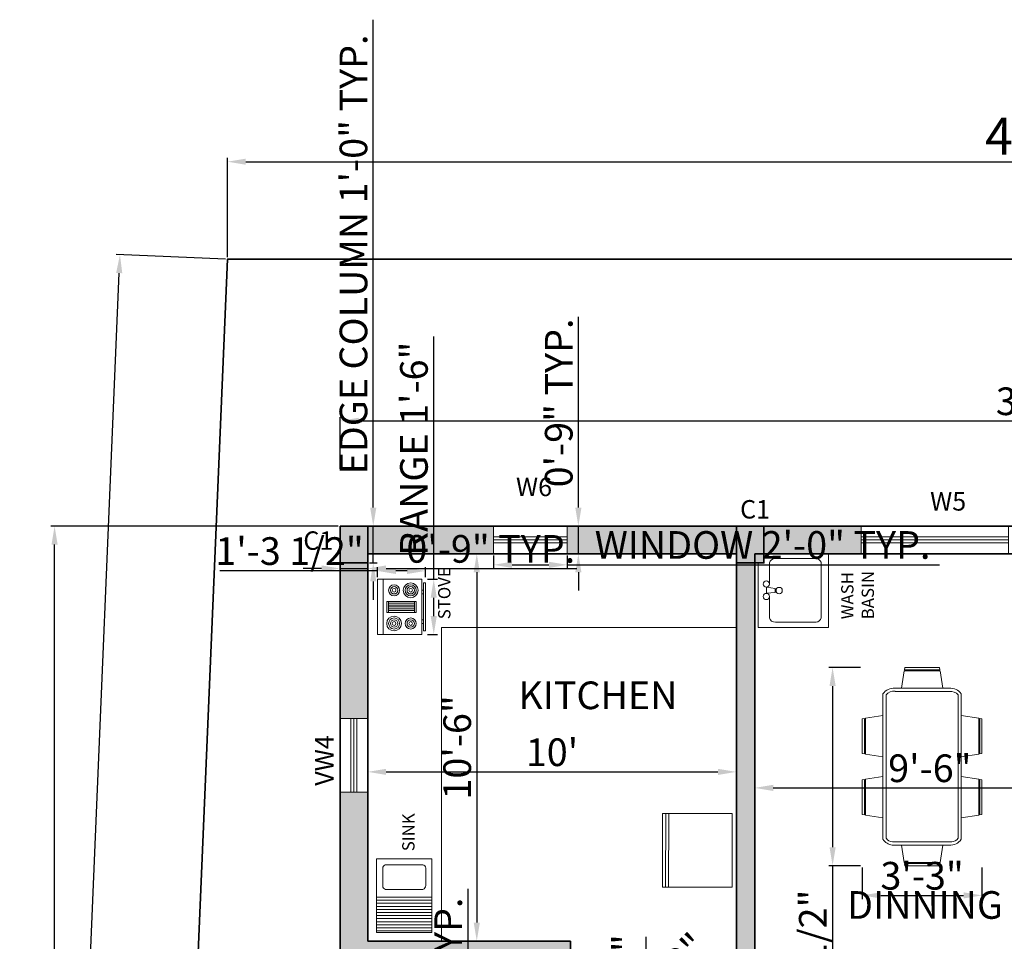
# Model space of a CAD drawing. Units: inches. Extents: x 4312 to 4955, y 6030 to 6717.
# Tile 4 of 5: x 4312 to 4632, y 6418 to 6717. Entities that reach past the tile are written whole.
import ezdxf

# ---------------------------------------------------------------- set-up
doc = ezdxf.new("R2010")
doc.units = ezdxf.units.IN
for name, color, linetype, lineweight in [('A-AREA-IDEN', 7, 'Continuous', 20), ('A-EQPM', 8, 'Continuous', 18), ('A-FLOR-CASE', 40, 'Continuous', 18), ('A-FLOR-FIXT', 9, 'Continuous', 18), ('A-FLOR-FIXT-PATT', 9, 'Continuous', 13), ('A-WALL', 7, 'Continuous', 35), ('C-PROP', 7, 'Continuous', 35), ('Dimensions', 112, 'Continuous', 13), ('Furniture', 30, 'Continuous', 18), ('Text', 30, 'Continuous', 18), ('Windows', 160, 'Continuous', 18)]:
    doc.layers.add(name, color=color, linetype=linetype, lineweight=lineweight)
doc.layers.add('A-WALL-PATT', color=251, linetype='Continuous', lineweight=13, true_color=0x636466)
doc.layers.add('Column', color=52, linetype='Continuous', lineweight=35, true_color=0xc8c92d)
doc.styles.get("Standard").update_dxf_attribs({"font": 'arial.ttf'})
doc.dimstyles.new('ISO-25', dxfattribs={"dimtxt": 9, "dimasz": 6, "dimexe": 1.25, "dimexo": 0.625, "dimtad": 1, "dimdec": 1, "dimlunit": 3, "dimtxsty": 'Standard', "dimcen": 2.5, "dimadec": 0, "dimazin": 0, "dimtfac": 1, "dimtdec": 1, "dimtmove": 0, "dimatfit": 3, "dimfxl": 1, "dimarcsym": 0})

# ---------------------------------------------------------------- blocks, each defined once
blk = doc.blocks.new('W')
at = {"layer": 'Windows'}
for p, q in [((4457.75, 6177.72), (4457.75, 6168.72)), ((4505.75, 6177.72), (4505.75, 6168.72)), ((4457.75, 6174.22), (4505.75, 6174.22)), ((4457.75, 6173.22), (4505.75, 6173.22)), ((4457.75, 6172.22), (4505.75, 6172.22))]:
    blk.add_line(p, q, dxfattribs=at)
blk = doc.blocks.new('KW')
at = {"layer": 'Windows'}
for p, q in [((4466.02, 6552.72), (4466.02, 6543.72)), ((4490.02, 6552.72), (4490.02, 6543.72)), ((4466.02, 6549.22), (4490.02, 6549.22)), ((4466.02, 6548.22), (4490.02, 6548.22)), ((4466.02, 6547.22), (4490.02, 6547.22))]:
    blk.add_line(p, q, dxfattribs=at)
blk = doc.blocks.new('*D9')
at = {"layer": 'Defpoints', "color": 0, "transparency": 16777216}
for p in [(4460.55, 6543.72), (4460.55, 6417.72), (4460.55, 6417.72)]:
    blk.add_point(p, dxfattribs=at)
at = {"layer": 'Dimensions', "color": 0, "lineweight": -2, "transparency": 16777216}
for p, q in [((4461.17, 6543.72), (4461.8, 6543.72)), ((4460.55, 6537.72), (4460.55, 6423.72)), ((4461.17, 6417.72), (4461.8, 6417.72))]:
    blk.add_line(p, q, dxfattribs=at)
at = {"layer": 'Dimensions', "color": 0, "transparency": 16777216}
for points in [[(4459.55, 6537.72), (4461.55, 6537.72), (4460.55, 6543.72)], [(4459.55, 6423.72), (4461.55, 6423.72), (4460.55, 6417.72)]]:
    blk.add_solid(points, dxfattribs=at)
at = {"layer": 'Dimensions', "color": 0, "transparency": 16777216, "insert": (4455.33, 6480.72), "char_height": 9, "attachment_point": 5, "rotation": 90}
blk.add_mtext('10\'-6"', dxfattribs=at)
blk = doc.blocks.new('*D10')
at = {"layer": 'Defpoints', "color": 0, "transparency": 16777216}
for p in [(4425.05, 6472.76), (4545.05, 6472.76), (4545.05, 6472.76)]:
    blk.add_point(p, dxfattribs=at)
at = {"layer": 'Dimensions', "color": 0, "lineweight": -2, "transparency": 16777216}
for p, q in [((4425.05, 6473.38), (4425.05, 6474.01)), ((4431.05, 6472.76), (4539.05, 6472.76)), ((4545.05, 6473.38), (4545.05, 6474.01))]:
    blk.add_line(p, q, dxfattribs=at)
at = {"layer": 'Dimensions', "color": 0, "transparency": 16777216}
for points in [[(4431.05, 6473.76), (4431.05, 6471.76), (4425.05, 6472.76)], [(4539.05, 6473.76), (4539.05, 6471.76), (4545.05, 6472.76)]]:
    blk.add_solid(points, dxfattribs=at)
at = {"layer": 'Dimensions', "color": 0, "transparency": 16777216, "insert": (4485.05, 6477.98), "char_height": 9, "attachment_point": 5}
blk.add_mtext("10'", dxfattribs=at)
blk = doc.blocks.new('*D11')
at = {"layer": 'Defpoints', "color": 0, "transparency": 16777216}
for p in [(4551.05, 6471.59), (4665.05, 6471.59), (4665.05, 6467.55)]:
    blk.add_point(p, dxfattribs=at)
at = {"layer": 'Dimensions', "color": 0, "lineweight": -2, "transparency": 16777216}
for p, q in [((4551.05, 6470.96), (4551.05, 6466.3)), ((4665.05, 6470.96), (4665.05, 6466.3)), ((4557.05, 6467.55), (4659.05, 6467.55))]:
    blk.add_line(p, q, dxfattribs=at)
at = {"layer": 'Dimensions', "color": 0, "transparency": 16777216}
for points in [[(4557.05, 6468.55), (4557.05, 6466.55), (4551.05, 6467.55)], [(4659.05, 6468.55), (4659.05, 6466.55), (4665.05, 6467.55)]]:
    blk.add_solid(points, dxfattribs=at)
at = {"layer": 'Dimensions', "color": 0, "transparency": 16777216, "insert": (4608.05, 6472.77), "char_height": 9, "attachment_point": 5}
blk.add_mtext('9\'-6"', dxfattribs=at)
blk = doc.blocks.new('Range-Oven - 30 in top')
for p, q in [((0, -3), (30, -3)), ((12, -6), (18, -6)), ((13, -20), (13, -6)), ((14, -6), (14, -20)), ((15, -20), (15, -6)), ((16, -6), (16, -20)), ((17, -20), (17, -6)), ((18, -20), (12, -20)), ((6, -24), (6, -25)), ((8, -25), (8, -24)), ((22, -25), (22, -24)), ((24, -24), (24, -25))]:
    blk.add_line(p, q)
for points in [[(0, -24), (0, 0), (30, 0), (30, -24)], [(12, -21), (12, -5), (18, -5), (18, -21)], [(2, -26), (2, -25), (28, -25), (28, -26)]]:
    blk.add_lwpolyline(points, close=True)
for centre, radius in [((6, -9), 4), ((6, -9), 3), ((6, -9), 2), ((6, -9), 1), ((24, -9), 3), ((24, -9), 2), ((24, -9), 1), ((6, -18), 3), ((6, -18), 2), ((24, -18), 4), ((24, -18), 3), ((24, -18), 2), ((6, -18), 1), ((24, -18), 1)]:
    blk.add_circle(centre, radius)
blk = doc.blocks.new('dinning')
for p, q in [((5019.18, 6524.81), (5018.3, 6519.14)), ((5019.18, 6524.81), (5030.85, 6524.81)), ((5019.35, 6525.87), (5019.24, 6525.17)), ((5030.79, 6525.17), (5019.24, 6525.17)), ((5019.35, 6525.87), (5030.68, 6525.87)), ((5030.79, 6525.17), (5030.68, 6525.87)), ((5031.73, 6519.14), (5030.85, 6524.81)), ((5039.01, 6524.81), (5038.13, 6519.14)), ((5039.02, 6524.81), (5050.68, 6524.81)), ((5039.18, 6525.87), (5039.07, 6525.17)), ((5050.62, 6525.17), (5039.07, 6525.17)), ((5039.18, 6525.87), (5050.51, 6525.87)), ((5050.62, 6525.17), (5050.51, 6525.87)), ((5051.56, 6519.14), (5050.68, 6524.81)), ((5058.57, 6519.15), (5011.29, 6519.15)), ((5058.25, 6518.15), (5011.62, 6518.15)), ((5003.77, 6512.23), (5009.43, 6513.11)), ((5009.43, 6515.21), (5009.43, 6497.59)), ((5010.43, 6515.26), (5010.43, 6497.59)), ((5059.43, 6496.76), (5059.43, 6516.04)), ((5060.43, 6496.7), (5060.43, 6515.21)), ((5066.1, 6512.23), (5060.43, 6513.11)), ((5002.7, 6512.06), (5003.41, 6512.17)), ((5002.7, 6512.06), (5002.7, 6500.73)), ((5003.41, 6500.62), (5003.41, 6512.17)), ((5003.77, 6512.23), (5003.77, 6500.56)), ((5066.09, 6512.23), (5066.09, 6500.56)), ((5067.16, 6512.06), (5066.45, 6512.17)), ((5066.45, 6500.62), (5066.45, 6512.17)), ((5067.16, 6512.06), (5067.16, 6500.73)), ((5003.41, 6500.62), (5002.7, 6500.73)), ((5009.43, 6499.68), (5003.77, 6500.56)), ((5060.43, 6499.68), (5066.09, 6500.56)), ((5066.45, 6500.62), (5067.16, 6500.73)), ((5011.62, 6494.65), (5058.25, 6494.65)), ((5011.29, 6493.65), (5058.57, 6493.65)), ((5019.18, 6487.98), (5018.3, 6493.65)), ((5031.73, 6493.65), (5030.85, 6487.98)), ((5039.01, 6487.98), (5038.13, 6493.65)), ((5051.56, 6493.65), (5050.68, 6487.98)), ((5019.18, 6487.98), (5030.85, 6487.98)), ((5019.35, 6486.92), (5019.24, 6487.63)), ((5030.79, 6487.63), (5019.24, 6487.63)), ((5030.79, 6487.63), (5030.68, 6486.92)), ((5039.02, 6487.98), (5050.68, 6487.98)), ((5039.18, 6486.92), (5039.07, 6487.63)), ((5050.62, 6487.63), (5039.07, 6487.63)), ((5050.62, 6487.63), (5050.51, 6486.92)), ((5019.35, 6486.92), (5030.68, 6486.92)), ((5039.18, 6486.92), (5050.51, 6486.92))]:
    blk.add_line(p, q)
for centre, radius, start, end in [((5013.59, 6515.65), 4.18, 123.3176, 186.0843), ((5013.59, 6515.65), 3.18, 128.372, 186.976), ((5056.27, 6515.65), 3.18, 6.976, 51.628), ((5056.27, 6515.65), 4.18, 353.9157, 56.6824), ((5013.59, 6497.14), 4.18, 173.9157, 236.6824), ((5013.61, 6497.16), 3.21, 172.3391, 231.5588), ((5056.27, 6497.14), 3.18, 308.372, 353.024), ((5056.27, 6497.14), 4.18, 303.3176, 353.9157)]:
    blk.add_arc(centre, radius, start, end)
blk = doc.blocks.new('*D38')
at = {"layer": 'Defpoints', "color": 0, "transparency": 16777216}
for p in [(4860.05, 6586.94), (4416.05, 6570.77), (4860.05, 6570.77)]:
    blk.add_point(p, dxfattribs=at)
at = {"layer": 'Dimensions', "color": 0, "lineweight": -2, "transparency": 16777216}
for p, q in [((4416.05, 6571.39), (4416.05, 6588.19)), ((4422.05, 6586.94), (4854.05, 6586.94)), ((4860.05, 6571.39), (4860.05, 6588.19))]:
    blk.add_line(p, q, dxfattribs=at)
at = {"layer": 'Dimensions', "color": 0, "transparency": 16777216}
for points in [[(4422.05, 6587.94), (4422.05, 6585.94), (4416.05, 6586.94)], [(4854.05, 6587.94), (4854.05, 6585.94), (4860.05, 6586.94)]]:
    blk.add_solid(points, dxfattribs=at)
at = {"layer": 'Dimensions', "color": 0, "transparency": 16777216, "insert": (4638.05, 6592.16), "char_height": 9, "attachment_point": 5}
blk.add_mtext("37'", dxfattribs=at)
blk = doc.blocks.new('*D40')
at = {"layer": 'Defpoints', "color": 0, "transparency": 16777216}
for p in [(4895.36, 6671.27), (4379.36, 6639.55), (4895.36, 6639.55)]:
    blk.add_point(p, dxfattribs=at)
at = {"layer": 'Dimensions', "color": 0, "lineweight": -2, "transparency": 16777216}
for p, q in [((4379.36, 6640.17), (4379.36, 6672.52)), ((4385.36, 6671.27), (4889.36, 6671.27)), ((4895.36, 6640.17), (4895.36, 6672.52))]:
    blk.add_line(p, q, dxfattribs=at)
at = {"layer": 'Dimensions', "color": 0, "transparency": 16777216}
for points in [[(4385.36, 6672.27), (4385.36, 6670.27), (4379.36, 6671.27)], [(4889.36, 6672.27), (4889.36, 6670.27), (4895.36, 6671.27)]]:
    blk.add_solid(points, dxfattribs=at)
at = {"layer": 'Dimensions', "color": 0, "transparency": 16777216, "insert": (4637.36, 6678.02), "char_height": 12, "attachment_point": 5}
blk.add_mtext("43'", dxfattribs=at)
blk = doc.blocks.new('*D43')
at = {"layer": 'Defpoints', "color": 0, "transparency": 16777216}
for p in [(4344.4, 6641.02), (4379.36, 6639.55), (4355.36, 6070.55)]:
    blk.add_point(p, dxfattribs=at)
at = {"layer": 'Dimensions', "color": 0, "lineweight": -2, "transparency": 16777216}
for p, q in [((4378.74, 6639.57), (4343.16, 6641.08)), ((4320.66, 6078.02), (4344.15, 6635.03)), ((4354.74, 6070.57), (4319.16, 6072.08))]:
    blk.add_line(p, q, dxfattribs=at)
at = {"layer": 'Dimensions', "color": 0, "transparency": 16777216}
for points in [[(4343.15, 6635.07), (4345.15, 6634.99), (4344.4, 6641.02)], [(4319.66, 6078.06), (4321.66, 6077.98), (4320.4, 6072.02)]]:
    blk.add_solid(points, dxfattribs=at)
at = {"layer": 'Dimensions', "color": 0, "transparency": 16777216, "insert": (4325.68, 6356.81), "char_height": 12, "attachment_point": 5, "rotation": 87.5847}
blk.add_mtext('47\'-5.5"', dxfattribs=at)
blk = doc.blocks.new('COLUMN-9X12-EDGE')
h = blk.add_hatch(color=256)
h.dxf.hatch_style = 1
h.paths.add_polyline_path([(9, 12), (0, 12), (0, 0), (9, 0)])
blk.add_lwpolyline([(9, 0), (0, 0)])
blk = doc.blocks.new('*D53')
at = {"layer": 'Defpoints', "color": 0, "transparency": 16777216}
for p in [(4425.05, 6552.72), (4426.85, 6552.72), (4425.05, 6540.72)]:
    blk.add_point(p, dxfattribs=at)
at = {"layer": 'Dimensions', "color": 0, "lineweight": -2, "transparency": 16777216}
for p, q in [((4426.85, 6558.72), (4426.85, 6717.46)), ((4425.67, 6552.72), (4428.1, 6552.72)), ((4426.85, 6540.72), (4426.85, 6552.72)), ((4425.67, 6540.72), (4428.1, 6540.72)), ((4426.85, 6534.72), (4426.85, 6528.72))]:
    blk.add_line(p, q, dxfattribs=at)
at = {"layer": 'Dimensions', "color": 0, "transparency": 16777216}
for points in [[(4425.85, 6558.72), (4427.85, 6558.72), (4426.85, 6552.72)], [(4425.85, 6534.72), (4427.85, 6534.72), (4426.85, 6540.72)]]:
    blk.add_solid(points, dxfattribs=at)
at = {"layer": 'Dimensions', "color": 0, "transparency": 16777216, "insert": (4421.57, 6641.09), "char_height": 9, "attachment_point": 5, "rotation": 90}
blk.add_mtext('EDGE COLUMN 1\'-0" TYP.', dxfattribs=at)
blk = doc.blocks.new('*D54')
at = {"layer": 'Defpoints', "color": 0, "transparency": 16777216}
for p in [(4416.05, 6540.72), (4425.05, 6540.72), (4425.05, 6538.92)]:
    blk.add_point(p, dxfattribs=at)
at = {"layer": 'Dimensions', "color": 0, "lineweight": -2, "transparency": 16777216}
for p, q in [((4410.05, 6538.92), (4404.05, 6538.92)), ((4416.05, 6540.1), (4416.05, 6537.67)), ((4416.05, 6538.92), (4425.05, 6538.92)), ((4425.05, 6540.1), (4425.05, 6537.67)), ((4431.05, 6538.92), (4493.16, 6538.92))]:
    blk.add_line(p, q, dxfattribs=at)
at = {"layer": 'Dimensions', "color": 0, "transparency": 16777216}
for points in [[(4410.05, 6539.92), (4410.05, 6537.92), (4416.05, 6538.92)], [(4431.05, 6539.92), (4431.05, 6537.92), (4425.05, 6538.92)]]:
    blk.add_solid(points, dxfattribs=at)
at = {"layer": 'Dimensions', "color": 0, "transparency": 16777216, "insert": (4465.1, 6544.14), "char_height": 9, "attachment_point": 5}
blk.add_mtext('0\'-9" TYP.', dxfattribs=at)
blk = doc.blocks.new('*D63')
at = {"layer": 'Defpoints', "color": 0, "transparency": 16777216}
for p in [(4466.02, 6543.72), (4490.02, 6543.72), (4490.02, 6540.12)]:
    blk.add_point(p, dxfattribs=at)
at = {"layer": 'Dimensions', "color": 0, "lineweight": -2, "transparency": 16777216}
for p, q in [((4466.02, 6543.1), (4466.02, 6538.87)), ((4490.02, 6543.1), (4490.02, 6538.87)), ((4472.02, 6540.12), (4484.02, 6540.12)), ((4490.02, 6540.12), (4611.16, 6540.12))]:
    blk.add_line(p, q, dxfattribs=at)
at = {"layer": 'Dimensions', "color": 0, "transparency": 16777216}
for points in [[(4472.02, 6541.12), (4472.02, 6539.12), (4466.02, 6540.12)], [(4484.02, 6541.12), (4484.02, 6539.12), (4490.02, 6540.12)]]:
    blk.add_solid(points, dxfattribs=at)
at = {"layer": 'Dimensions', "color": 0, "transparency": 16777216, "insert": (4553.59, 6545.41), "char_height": 9, "attachment_point": 5}
blk.add_mtext('WINDOW 2\'-0" TYP.', dxfattribs=at)
blk = doc.blocks.new('*D64')
at = {"layer": 'Defpoints', "color": 0, "transparency": 16777216}
for p in [(4490.02, 6552.72), (4493.62, 6552.72), (4490.02, 6543.72)]:
    blk.add_point(p, dxfattribs=at)
at = {"layer": 'Dimensions', "color": 0, "lineweight": -2, "transparency": 16777216}
for p, q in [((4493.62, 6558.72), (4493.62, 6620.83)), ((4490.65, 6552.72), (4494.87, 6552.72)), ((4493.62, 6543.72), (4493.62, 6552.72)), ((4490.65, 6543.72), (4494.87, 6543.72)), ((4493.62, 6537.72), (4493.62, 6531.72))]:
    blk.add_line(p, q, dxfattribs=at)
at = {"layer": 'Dimensions', "color": 0, "transparency": 16777216}
for points in [[(4492.62, 6558.72), (4494.62, 6558.72), (4493.62, 6552.72)], [(4492.62, 6537.72), (4494.62, 6537.72), (4493.62, 6543.72)]]:
    blk.add_solid(points, dxfattribs=at)
at = {"layer": 'Dimensions', "color": 0, "transparency": 16777216, "insert": (4488.4, 6592.78), "char_height": 9, "attachment_point": 5, "rotation": 90}
blk.add_mtext('0\'-9" TYP.', dxfattribs=at)
blk = doc.blocks.new('*D70')
at = {"layer": 'Defpoints', "color": 0, "transparency": 16777216}
for p in [(4512.05, 6387.72), (4515.65, 6387.72), (4512.05, 6363.72)]:
    blk.add_point(p, dxfattribs=at)
at = {"layer": 'Dimensions', "color": 0, "lineweight": -2, "transparency": 16777216}
for p, q in [((4515.65, 6387.72), (4515.65, 6419.05)), ((4512.67, 6387.72), (4516.9, 6387.72)), ((4515.65, 6369.72), (4515.65, 6381.72)), ((4512.67, 6363.72), (4516.9, 6363.72))]:
    blk.add_line(p, q, dxfattribs=at)
at = {"layer": 'Dimensions', "color": 0, "transparency": 16777216}
for points in [[(4514.65, 6381.72), (4516.65, 6381.72), (4515.65, 6387.72)], [(4514.65, 6369.72), (4516.65, 6369.72), (4515.65, 6363.72)]]:
    blk.add_solid(points, dxfattribs=at)
at = {"layer": 'Dimensions', "color": 0, "transparency": 16777216, "insert": (4510.43, 6406.39), "char_height": 9, "attachment_point": 5, "rotation": 90}
blk.add_mtext('2\'-0"', dxfattribs=at)
blk = doc.blocks.new('*D73')
at = {"layer": 'Defpoints', "color": 0, "transparency": 16777216}
for p in [(4447.05, 6327.89), (4457.7, 6327.89), (4447.05, 6256.83)]:
    blk.add_point(p, dxfattribs=at)
at = {"layer": 'Dimensions', "color": 0, "lineweight": -2, "transparency": 16777216}
for p, q in [((4457.7, 6327.89), (4457.7, 6434.68)), ((4447.67, 6327.89), (4458.95, 6327.89)), ((4457.7, 6262.83), (4457.7, 6321.89)), ((4447.67, 6256.83), (4458.95, 6256.83))]:
    blk.add_line(p, q, dxfattribs=at)
at = {"layer": 'Dimensions', "color": 0, "transparency": 16777216}
for points in [[(4456.7, 6321.89), (4458.7, 6321.89), (4457.7, 6327.89)], [(4456.7, 6262.83), (4458.7, 6262.83), (4457.7, 6256.83)]]:
    blk.add_solid(points, dxfattribs=at)
at = {"layer": 'Dimensions', "color": 0, "transparency": 16777216, "insert": (4452.42, 6384.28), "char_height": 9, "attachment_point": 5, "rotation": 90}
blk.add_mtext('SOFA 5\'-11" TYP.', dxfattribs=at)
blk = doc.blocks.new('*D81')
at = {"layer": 'Defpoints', "color": 0, "transparency": 16777216}
for p in [(4443.84, 6535.43), (4446.54, 6535.43), (4443.84, 6517.43)]:
    blk.add_point(p, dxfattribs=at)
at = {"layer": 'Dimensions', "color": 0, "lineweight": -2, "transparency": 16777216}
for p, q in [((4446.54, 6535.43), (4446.54, 6614.35)), ((4444.47, 6535.43), (4447.79, 6535.43)), ((4446.54, 6523.43), (4446.54, 6529.43)), ((4444.47, 6517.43), (4447.79, 6517.43))]:
    blk.add_line(p, q, dxfattribs=at)
at = {"layer": 'Dimensions', "color": 0, "transparency": 16777216}
for points in [[(4445.54, 6529.43), (4447.54, 6529.43), (4446.54, 6535.43)], [(4445.54, 6523.43), (4447.54, 6523.43), (4446.54, 6517.43)]]:
    blk.add_solid(points, dxfattribs=at)
at = {"layer": 'Dimensions', "color": 0, "transparency": 16777216, "insert": (4441.26, 6577.89), "char_height": 9, "attachment_point": 5, "rotation": 90}
blk.add_mtext('RANGE 1\'-6"', dxfattribs=at)
blk = doc.blocks.new('*D82')
at = {"layer": 'Defpoints', "color": 0, "transparency": 16777216}
for p in [(4428.24, 6538.13), (4428.24, 6535.43), (4443.84, 6535.43)]:
    blk.add_point(p, dxfattribs=at)
at = {"layer": 'Dimensions', "color": 0, "lineweight": -2, "transparency": 16777216}
for p, q in [((4428.24, 6536.06), (4428.24, 6539.38)), ((4443.84, 6536.06), (4443.84, 6539.38)), ((4428.24, 6538.13), (4376.94, 6538.13)), ((4437.84, 6538.13), (4434.24, 6538.13))]:
    blk.add_line(p, q, dxfattribs=at)
at = {"layer": 'Dimensions', "color": 0, "transparency": 16777216}
for points in [[(4434.24, 6539.13), (4434.24, 6537.13), (4428.24, 6538.13)], [(4437.84, 6539.13), (4437.84, 6537.13), (4443.84, 6538.13)]]:
    blk.add_solid(points, dxfattribs=at)
at = {"layer": 'Dimensions', "color": 0, "transparency": 16777216, "insert": (4399.59, 6543.42), "char_height": 9, "attachment_point": 5}
blk.add_mtext('1\'-3 1/2"', dxfattribs=at)
blk = doc.blocks.new('*D83')
at = {"layer": 'Defpoints', "color": 0, "transparency": 16777216}
for p in [(4586.05, 6506.69), (4576.38, 6442.24), (4586.05, 6442.24)]:
    blk.add_point(p, dxfattribs=at)
at = {"layer": 'Dimensions', "color": 0, "lineweight": -2, "transparency": 16777216}
for p, q in [((4585.42, 6506.69), (4575.13, 6506.69)), ((4576.38, 6500.69), (4576.38, 6448.24)), ((4585.42, 6442.24), (4575.13, 6442.24)), ((4576.38, 6442.24), (4576.38, 6315.1))]:
    blk.add_line(p, q, dxfattribs=at)
at = {"layer": 'Dimensions', "color": 0, "transparency": 16777216}
for points in [[(4575.38, 6500.69), (4577.38, 6500.69), (4576.38, 6506.69)], [(4575.38, 6448.24), (4577.38, 6448.24), (4576.38, 6442.24)]]:
    blk.add_solid(points, dxfattribs=at)
at = {"layer": 'Dimensions', "color": 0, "transparency": 16777216, "insert": (4571.1, 6375.67), "char_height": 9, "attachment_point": 5, "rotation": 90}
blk.add_mtext('DINING SET 5\'-4 1/2"', dxfattribs=at)
blk = doc.blocks.new('*D84')
at = {"layer": 'Defpoints', "color": 0, "transparency": 16777216}
for p in [(4586.05, 6442.24), (4625, 6442.24), (4625, 6432.57)]:
    blk.add_point(p, dxfattribs=at)
at = {"layer": 'Dimensions', "color": 0, "lineweight": -2, "transparency": 16777216}
for p, q in [((4586.05, 6441.61), (4586.05, 6431.32)), ((4625, 6441.61), (4625, 6431.32)), ((4592.05, 6432.57), (4619, 6432.57))]:
    blk.add_line(p, q, dxfattribs=at)
at = {"layer": 'Dimensions', "color": 0, "transparency": 16777216}
for points in [[(4592.05, 6433.57), (4592.05, 6431.57), (4586.05, 6432.57)], [(4619, 6433.57), (4619, 6431.57), (4625, 6432.57)]]:
    blk.add_solid(points, dxfattribs=at)
at = {"layer": 'Dimensions', "color": 0, "transparency": 16777216, "insert": (4605.52, 6437.79), "char_height": 9, "attachment_point": 5}
blk.add_mtext('3\'-3"', dxfattribs=at)
blk = doc.blocks.new('*D90')
at = {"layer": 'Defpoints', "color": 0, "transparency": 16777216}
for p in [(4323.11, 6552.72), (4416.05, 6552.72), (4368.05, 6087.72)]:
    blk.add_point(p, dxfattribs=at)
at = {"layer": 'Dimensions', "color": 0, "lineweight": -2, "transparency": 16777216}
for p, q in [((4415.42, 6552.72), (4321.86, 6552.72)), ((4323.11, 6093.72), (4323.11, 6546.72)), ((4367.42, 6087.72), (4321.86, 6087.72))]:
    blk.add_line(p, q, dxfattribs=at)
at = {"layer": 'Dimensions', "color": 0, "transparency": 16777216}
for points in [[(4322.11, 6546.72), (4324.11, 6546.72), (4323.11, 6552.72)], [(4322.11, 6093.72), (4324.11, 6093.72), (4323.11, 6087.72)]]:
    blk.add_solid(points, dxfattribs=at)
at = {"layer": 'Dimensions', "color": 0, "transparency": 16777216, "insert": (4317.89, 6320.22), "char_height": 9, "attachment_point": 5, "rotation": 90}
blk.add_mtext('38\'-9"', dxfattribs=at)
blk = doc.blocks.new('*D97')
at = {"layer": 'Defpoints', "color": 0, "transparency": 16777216}
for p in [(4505.02, 6380.69), (4488.05, 6363.72)]:
    blk.add_point(p, dxfattribs=at)
at = {"layer": 'Dimensions', "color": 0, "lineweight": -2, "transparency": 16777216}
for p, q in [((4537.4, 6413.07), (4509.26, 6384.94)), ((4488.05, 6363.72), (4505.02, 6380.69))]:
    blk.add_line(p, q, dxfattribs=at)
at = {"layer": 'Dimensions', "color": 0, "transparency": 16777216}
blk.add_solid([(4508.56, 6385.64), (4509.97, 6384.23), (4505.02, 6380.69)], dxfattribs=at)
at = {"layer": 'Dimensions', "color": 0, "transparency": 16777216, "insert": (4521.76, 6404.82), "char_height": 9, "attachment_point": 5, "rotation": 44.9998}
blk.add_mtext('R2\'-0"', dxfattribs=at)

msp = doc.modelspace()

# ---------------------------------------------------------------- hatches: boundary and pattern name
at = {"layer": 'A-FLOR-FIXT-PATT'}
h = msp.add_hatch(dxfattribs=at)
h.set_pattern_fill('ANSI31', color=256, scale=0.314961, angle=-45, style=0)
h.paths.add_polyline_path([(4427.93, 6420.52), (4445.93, 6420.52), (4445.93, 6432.52), (4427.93, 6432.52)])
at = {"layer": 'A-WALL-PATT'}
h = msp.add_hatch(color=256, dxfattribs=at)
h.dxf.hatch_style = 1
h.paths.add_polyline_path([(4466.02, 6552.72), (4425.05, 6552.72), (4425.05, 6543.72), (4466.02, 6543.72)])
h = msp.add_hatch(color=256, dxfattribs=at)
h.dxf.hatch_style = 1
h.paths.add_polyline_path([(4545.13, 6552.72), (4490.02, 6552.72), (4490.02, 6543.72), (4545.13, 6543.72)])
h = msp.add_hatch(color=256, dxfattribs=at)
h.dxf.hatch_style = 1
h.paths.add_polyline_path([(4585.64, 6552.72), (4554.13, 6552.72), (4554.13, 6543.72), (4585.64, 6543.72)])
h = msp.add_hatch(color=256, dxfattribs=at)
h.dxf.hatch_style = 1
h.paths.add_polyline_path([(4425.05, 6540.72), (4416.05, 6540.72), (4416.05, 6490.16), (4425.05, 6490.16)])
h = msp.add_hatch(color=256, dxfattribs=at)
h.dxf.hatch_style = 1
h.paths.add_polyline_path([(4551.05, 6540.72), (4545.05, 6540.72), (4545.05, 6411.72), (4551.05, 6411.72)])
h = msp.add_hatch(color=256, dxfattribs=at)
h.dxf.hatch_style = 1
h.paths.add_polyline_path([(4425.05, 6466.16), (4416.05, 6466.16), (4416.05, 6392.17), (4425.05, 6392.17), (4425.05, 6411.72), (4485.05, 6411.72), (4485.05, 6387.72), (4491.05, 6387.72), (4491.05, 6417.72), (4425.05, 6417.72)])
at = {"layer": 'Column'}
h = msp.add_hatch(color=256, dxfattribs=at)
h.dxf.hatch_style = 1
h.paths.add_polyline_path([(4554.05, 6540.72), (4554.05, 6543.72), (4554.05, 6552.72), (4545.05, 6552.72), (4545.05, 6540.72), (4551.05, 6540.72)])

# ---------------------------------------------------------------- linework, layer by layer
at = {"layer": 'A-EQPM'}
for p, q in [((4521.05, 6459.2), (4521, 6435.2)), ((4543.67, 6459.2), (4521.05, 6459.2)), ((4522.05, 6459.2), (4522, 6435.2)), ((4523.05, 6459.2), (4523, 6435.2)), ((4543.67, 6459.2), (4543.67, 6435.2)), ((4545.05, 6459.2), (4545.05, 6459.2)), ((4521, 6435.2), (4543.67, 6435.2))]:
    msp.add_line(p, q, dxfattribs=at)
at = {"layer": 'A-FLOR-CASE'}
for p, q in [((4575.05, 6519.72), (4575.05, 6543.72)), ((4552.19, 6540.72), (4552.19, 6519.72)), ((4449.05, 6417.72), (4449.05, 6519.72)), ((4449.05, 6519.72), (4545.05, 6519.72)), ((4552.19, 6519.72), (4575.05, 6519.72))]:
    msp.add_line(p, q, dxfattribs=at)
at = {"layer": 'A-FLOR-FIXT'}
for points in [[(4570.94, 6542.18), (4557.61, 6542.18, 0.355496), (4555.86, 6540.75), (4555.86, 6533.87)], [(4555.86, 6529.82), (4555.86, 6522.89, 0.38014), (4557.77, 6521.47), (4571.02, 6521.47, 0.335385), (4572.63, 6522.9), (4572.63, 6540.95, 0.335385), (4570.86, 6542.18)]]:
    msp.add_lwpolyline(points, format="xyb", dxfattribs=at)
for points in [[(4554.84, 6530.85), (4557.69, 6531.12), (4557.69, 6532.46), (4554.84, 6532.85)], [(4427.93, 6420.52), (4427.93, 6444.52), (4445.93, 6444.52), (4445.93, 6420.52)]]:
    msp.add_lwpolyline(points, close=True, dxfattribs=at)
msp.add_lwpolyline([(4442.97, 6434.52, 0.38014), (4443.93, 6435.81), (4443.93, 6441.44, 0.335385), (4442.96, 6442.52), (4430.76, 6442.52, 0.335385), (4429.93, 6441.33), (4429.93, 6435.71, 0.355496), (4430.89, 6434.52)], format="xyb", close=True, dxfattribs=at)
for centre in [(4554.84, 6533.87), (4558.98, 6531.75), (4554.84, 6529.82)]:
    msp.add_circle(centre, 1.02, dxfattribs=at)
at = {"layer": 'A-WALL'}
for p, q in [((4416.05, 6223.72), (4416.05, 6552.72)), ((4416.05, 6552.72), (4860.05, 6552.72)), ((4425.05, 6417.72), (4425.05, 6552.72)), ((4545.05, 6552.72), (4545.05, 6411.72)), ((4425.05, 6543.72), (4545.05, 6543.72)), ((4551.05, 6543.72), (4551.05, 6411.72)), ((4551.05, 6543.72), (4851.05, 6543.72)), ((4425.05, 6417.72), (4491.05, 6417.72)), ((4491.05, 6387.72), (4491.05, 6417.72))]:
    msp.add_line(p, q, dxfattribs=at)
at = {"layer": 'C-PROP'}
msp.add_lwpolyline([(4895.36, 6639.55), (4895.36, 6070.55), (4355.36, 6070.55), (4379.36, 6639.55)], close=True, dxfattribs=at)
at = {"layer": 'Column'}
msp.add_lwpolyline([(4554.05, 6552.72), (4554.05, 6540.72), (4545.05, 6540.72)], dxfattribs=at)

# ---------------------------------------------------------------- block references
at = {"layer": 'A-EQPM', "xscale": 0.6, "yscale": 0.6, "zscale": 0.6, "rotation": 90}
msp.add_blockref('Range-Oven - 30 in top', (4428.24, 6517.43), dxfattribs=at)
at = {"layer": 'Column'}
msp.add_blockref('COLUMN-9X12-EDGE', (4416.05, 6540.72), dxfattribs=at)
at = {"layer": 'Furniture', "rotation": 270}
msp.add_blockref('dinning', (-1900.87, 11509.39), dxfattribs=at)
at = {"layer": 'Windows'}
for name, p in [('KW', (0, 0)), ('W', (127.88, 375))]:
    msp.add_blockref(name, p, dxfattribs=at)
at = {"layer": 'Windows', "rotation": 270}
msp.add_blockref('KW', (-2127.68, 10956.19), dxfattribs=at)

# ---------------------------------------------------------------- texts
at = {"layer": 'A-AREA-IDEN', "char_height": 9, "attachment_point": 1, "rotation": 0.0025}
for s, insert in [('KITCHEN', (4474.11, 6502.16)), ('DINNING', (4581.1, 6433.95))]:
    msp.add_mtext_dynamic_manual_height_columns(s, width=10.4718, gutter_width=12.5, heights=[0], dxfattribs=dict(at, insert=insert))
at = {"layer": 'Text', "char_height": 6, "attachment_point": 1}
for s, insert in [('W6', (4473.32, 6568.46)), ('C1', (4546.26, 6561.18)), ('W5', (4608.14, 6563.76)), ('C1', (4404.09, 6551))]:
    msp.add_mtext_dynamic_manual_height_columns(s, width=4.4911, gutter_width=12.5, heights=[0], dxfattribs=dict(at, insert=insert))
at = {"layer": 'Text', "attachment_point": 1, "rotation": 90}
for s, width, insert, char_height in [('STOVE', 9.0664, (4447.97, 6522.41), 4), ('WASH\\PBASIN', 9.0664, (4579.18, 6522.41), 4), ('VW4', 19.9533, (4407.92, 6468.24), 6), ('SINK', 9.0664, (4436.29, 6446.94), 4)]:
    msp.add_mtext_dynamic_manual_height_columns(s, width=width, gutter_width=12.5, heights=[0], dxfattribs=dict(at, insert=insert, char_height=char_height))

# ---------------------------------------------------------------- dimensions: what is measured, and where the dimension line sits
at = {"layer": 'Dimensions'}
for base, p1, p2, angle, text, picture, middle in [((4426.85, 6552.72), (4425.05, 6540.72), (4425.05, 6552.72), 90, 'EDGE COLUMN <> TYP.', '*D53', (4421.57, 6641.09)), ((4493.62, 6552.72), (4490.02, 6543.72), (4490.02, 6552.72), 90, '<> TYP.', '*D64', (4488.4, 6592.78)), ((4446.54, 6535.43), (4443.84, 6517.43), (4443.84, 6535.43), 90, 'RANGE <>', '*D81', (4441.26, 6577.89)), ((4576.3781, 6442.2371), (4586.0462, 6506.6912), (4586.0462, 6442.2371), 270, 'DINING SET <>', '*D83', (4571.0996, 6375.6663)), ((4457.7, 6327.89), (4447.05, 6256.83), (4447.05, 6327.89), 90, 'SOFA <> TYP.', '*D73', (4452.42, 6384.28))]:
    dim = msp.add_linear_dim(base=base, p1=p1, p2=p2, angle=angle, text=text, dimstyle='ISO-25', override={"dimdec": 1, "dimlfac": 1, "dimrnd": 0, "dimzin": 1, "dimdsep": 46, "dimlunit": 4, "dimfrac": 2}, dxfattribs=at)
    dim.commit()
    dim.dimension.update_dxf_attribs({"geometry": picture, "text_midpoint": middle})
for base, p1, p2, override, picture, middle in [((4895.36, 6671.27), (4379.36, 6639.55), (4895.36, 6639.55), {"dimtxt": 12, "dimclrd": 0, "dimclre": 0, "dimclrt": 0}, '*D40', (4637.36, 6678.02)), ((4860.05, 6586.94), (4416.05, 6570.77), (4860.05, 6570.77), {"dimclrd": 0, "dimclre": 0, "dimclrt": 0}, '*D38', (4638.05, 6592.16)), ((4545.05, 6472.76), (4425.05, 6472.76), (4545.05, 6472.76), {"dimclrd": 0, "dimclre": 0, "dimclrt": 0}, '*D10', (4485.05, 6477.98)), ((4665.05, 6467.55), (4551.05, 6471.59), (4665.05, 6471.59), {"dimclrd": 0, "dimclre": 0, "dimclrt": 0}, '*D11', (4608.05, 6472.77)), ((4625.0019, 6432.569), (4586.0462, 6442.2371), (4625.0019, 6442.2371), {"dimdec": 1, "dimlfac": 1, "dimrnd": 0, "dimzin": 1, "dimdsep": 46, "dimlunit": 4, "dimfrac": 2}, '*D84', (4605.5241, 6437.7922))]:
    dim = msp.add_linear_dim(base=base, p1=p1, p2=p2, dimstyle='ISO-25', override=override, dxfattribs=at)
    dim.commit()
    dim.dimension.update_dxf_attribs({"geometry": picture, "text_midpoint": middle})
dim = msp.add_aligned_dim(p1=(4355.36, 6070.55), p2=(4379.36, 6639.55), distance=34.99, dimstyle='ISO-25', override={"dimtxt": 12, "dimclrd": 0, "dimclre": 0, "dimclrt": 0}, dxfattribs=at)
dim.commit()
dim.dimension.update_dxf_attribs({"geometry": '*D43', "text_midpoint": (4325.68, 6356.81)})
for base, p1, p2, text, picture, middle in [((4490.02, 6540.12), (4466.02, 6543.72), (4490.02, 6543.72), 'WINDOW <> TYP.', '*D63', (4553.59, 6545.41)), ((4425.05, 6538.92), (4416.05, 6540.72), (4425.05, 6540.72), '<> TYP.', '*D54', (4465.1, 6544.14))]:
    dim = msp.add_linear_dim(base=base, p1=p1, p2=p2, text=text, dimstyle='ISO-25', override={"dimdec": 1, "dimlfac": 1, "dimrnd": 0, "dimzin": 1, "dimdsep": 46, "dimlunit": 4, "dimfrac": 2}, dxfattribs=at)
    dim.commit()
    dim.dimension.update_dxf_attribs({"geometry": picture, "text_midpoint": middle})
for base, p1, p2, angle, override, picture, middle in [((4428.24, 6538.13), (4443.84, 6535.43), (4428.24, 6535.43), 180, {"dimdec": 1, "dimlfac": 1, "dimrnd": 0, "dimzin": 1, "dimdsep": 46, "dimlunit": 4, "dimfrac": 2}, '*D82', (4399.59, 6543.42)), ((4323.11, 6552.72), (4368.05, 6087.72), (4416.05, 6552.72), 90, {"dimdec": 1, "dimlfac": 1, "dimrnd": 0, "dimzin": 1, "dimdsep": 46, "dimlunit": 4, "dimfrac": 2}, '*D90', (4317.89, 6320.22)), ((4460.55, 6417.72), (4460.55, 6543.72), (4460.55, 6417.72), 90, {"dimclrd": 0, "dimclre": 0, "dimclrt": 0}, '*D9', (4455.33, 6480.72)), ((4515.65, 6387.72), (4512.05, 6363.72), (4512.05, 6387.72), 90, {"dimdec": 1, "dimlfac": 1, "dimrnd": 0, "dimzin": 1, "dimdsep": 46, "dimlunit": 4, "dimfrac": 2}, '*D70', (4510.43, 6406.39))]:
    dim = msp.add_linear_dim(base=base, p1=p1, p2=p2, angle=angle, dimstyle='ISO-25', override=override, dxfattribs=at)
    dim.commit()
    dim.dimension.update_dxf_attribs({"geometry": picture, "text_midpoint": middle})
dim = msp.add_radius_dim(center=(4488.05, 6363.72), mpoint=(4505.02, 6380.69), dimstyle='ISO-25', override={"dimdec": 1, "dimlfac": 1, "dimrnd": 0, "dimzin": 1, "dimdsep": 46, "dimlunit": 4, "dimfrac": 2}, dxfattribs=at)
dim.commit()
dim.dimension.update_dxf_attribs({"geometry": '*D97', "text_midpoint": (4521.76, 6404.82)})

doc.saveas('drawing.dxf')
